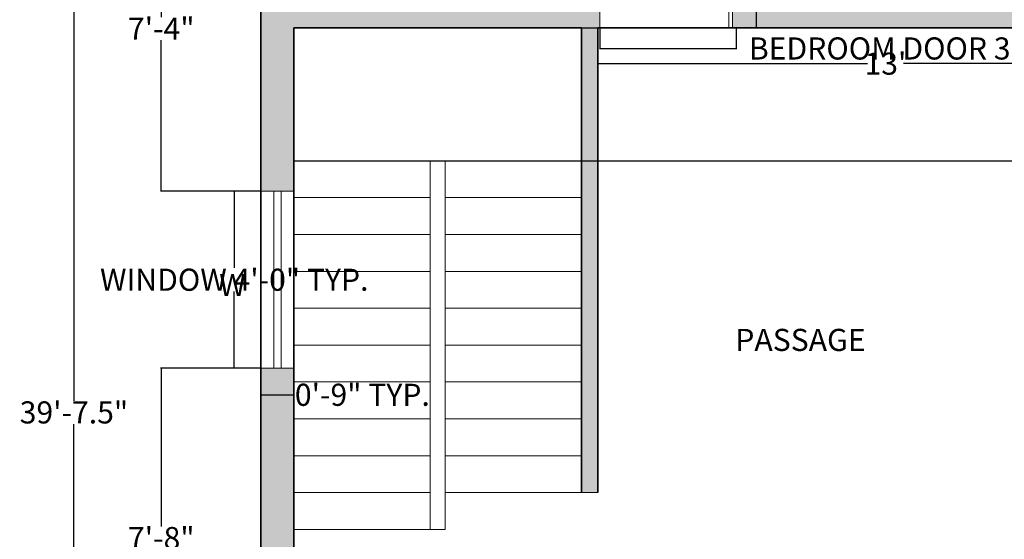
# Model space of a CAD drawing. Units: inches. Extents: x 302 to 1258, y 831 to 1373.
# Tile 2 of 13: x 302 to 569, y 1070 to 1211. Entities that reach past the tile are written whole.
import ezdxf

# ---------------------------------------------------------------- set-up
doc = ezdxf.new("R2010")
doc.units = ezdxf.units.IN
doc.header["$MEASUREMENT"] = 0
for name, color, linetype, lineweight in [('A-ANNO-DIMS', 2, 'Continuous', 18), ('A-ANNO-TEXT', 7, 'Continuous', 18), ('A-AREA-IDEN', 7, 'Continuous', 18), ('A-DOOR', 3, 'Continuous', 18), ('A-FLOR-STRS', 7, 'Continuous', 18), ('A-GLAZ', 4, 'Continuous', 18), ('A-WALL', 7, 'Continuous', 35), ('A-WALL-PATT', 251, 'Continuous', 13)]:
    doc.layers.add(name, color=color, linetype=linetype, lineweight=lineweight)
doc.styles.get("Standard").update_dxf_attribs({"font": 'arial.ttf'})
doc.dimstyles.get("Standard").update_dxf_attribs({"dimtxt": 6, "dimasz": 0.18, "dimexe": 0.18, "dimexo": 0.0625, "dimgap": 0.09, "dimtad": 0, "dimtih": 1, "dimtoh": 1, "dimdec": 1, "dimzin": 0, "dimdsep": 46, "dimlunit": 3, "dimtxsty": 'Standard', "dimcen": 0.09, "dimadec": 0, "dimazin": 0, "dimtfac": 1, "dimtdec": 1, "dimtofl": 0, "dimtmove": 0, "dimatfit": 3, "dimfxl": 1, "dimtolj": 1, "dimtzin": 0, "dimarcsym": 0})

# ---------------------------------------------------------------- blocks, each defined once
blk = doc.blocks.new('*D16')
at = {"layer": 'A-ANNO-DIMS', "color": 0, "lineweight": -2, "transparency": 16777216}
for p, q in [((459.17, 1208.76), (459.17, 1198.98)), ((615.17, 1208.76), (615.17, 1198.98)), ((459.35, 1199.16), (532.27, 1199.16)), ((614.99, 1199.16), (542.07, 1199.16))]:
    blk.add_line(p, q, dxfattribs=at)
at = {"layer": 'A-ANNO-DIMS', "color": 0, "transparency": 16777216}
for points in [[(459.35, 1199.19), (459.35, 1199.13), (459.17, 1199.16)], [(614.99, 1199.19), (614.99, 1199.13), (615.17, 1199.16)]]:
    blk.add_solid(points, dxfattribs=at)
at = {"layer": 'Defpoints', "color": 0, "transparency": 16777216}
for p in [(459.17, 1208.82), (615.17, 1208.82), (615.17, 1199.16)]:
    blk.add_point(p, dxfattribs=at)
at = {"layer": 'A-ANNO-DIMS', "color": 0, "transparency": 16777216, "insert": (537.17, 1199.16), "char_height": 6, "attachment_point": 5}
blk.add_mtext("\\A1;13'", dxfattribs=at)
blk = doc.blocks.new('*D32')
at = {"layer": 'A-ANNO-DIMS', "color": 0, "lineweight": -2, "transparency": 16777216}
for p, q in [((367.61, 1342.32), (316.79, 1342.32)), ((316.97, 1342.14), (316.97, 1107.72)), ((316.97, 867), (316.97, 1101.41)), ((367.61, 866.82), (316.79, 866.82))]:
    blk.add_line(p, q, dxfattribs=at)
at = {"layer": 'A-ANNO-DIMS', "color": 0, "transparency": 16777216}
for points in [[(316.94, 1342.14), (317, 1342.14), (316.97, 1342.32)], [(316.94, 867), (317, 867), (316.97, 866.82)]]:
    blk.add_solid(points, dxfattribs=at)
at = {"layer": 'Defpoints', "color": 0, "transparency": 16777216}
for p in [(367.67, 1342.32), (316.97, 866.82), (367.67, 866.82)]:
    blk.add_point(p, dxfattribs=at)
at = {"layer": 'A-ANNO-DIMS', "color": 0, "transparency": 16777216, "insert": (316.97, 1104.57), "char_height": 6, "attachment_point": 5}
blk.add_mtext('\\A1;39\'-7.5"', dxfattribs=at)
blk = doc.blocks.new('WINDOW-48IN')
for p, q in [((0, 0), (0, 9)), ((0, 9), (48, 9)), ((48, 9), (48, 0)), ((0, 5.5), (48, 5.5)), ((48, 3.5), (0, 3.5)), ((48, 0), (0, 0))]:
    blk.add_line(p, q)
blk = doc.blocks.new('DOOR-36IN-BEDROOM')
for p, q in [((35, 36), (35, 0)), ((36, 0), (36, 36)), ((36, 36), (36, 0)), ((0, 0), (0, 4.5)), ((36, 0), (0, 0)), ((37, 0), (36, 0))]:
    blk.add_line(p, q)
blk.add_arc((36, -0.32), 36.32, 90, 172.3719)
blk = doc.blocks.new('STAIR-RETURN-RUNS')
for p, q in [((0, 100), (78, 100)), ((37, 100), (37, 0)), ((41, 100), (41, 0)), ((0, 90), (37, 90)), ((41, 90), (78, 90)), ((0, 80), (37, 80)), ((41, 80), (78, 80)), ((0, 70), (37, 70)), ((41, 70), (78, 70)), ((0, 60), (37, 60)), ((41, 60), (78, 60)), ((0, 50), (37, 50)), ((41, 50), (78, 50)), ((0, 40), (37, 40)), ((41, 40), (78, 40)), ((0, 30), (37, 30)), ((41, 30), (78, 30)), ((0, 20), (37, 20)), ((41, 20), (78, 20)), ((0, 10), (37, 10)), ((41, 10), (82.5, 10)), ((0, 0), (41, 0))]:
    blk.add_line(p, q)
blk = doc.blocks.new('*D45')
at = {"layer": 'A-ANNO-DIMS', "color": 0, "lineweight": -2, "transparency": 16777216}
for p, q in [((367.61, 1164.55), (360.29, 1164.55)), ((360.47, 1164.37), (360.47, 1143.74)), ((360.47, 1116.73), (360.47, 1137.36)), ((367.61, 1116.55), (360.29, 1116.55))]:
    blk.add_line(p, q, dxfattribs=at)
at = {"layer": 'A-ANNO-DIMS', "color": 0, "transparency": 16777216}
for points in [[(360.44, 1164.37), (360.5, 1164.37), (360.47, 1164.55)], [(360.44, 1116.73), (360.5, 1116.73), (360.47, 1116.55)]]:
    blk.add_solid(points, dxfattribs=at)
at = {"layer": 'Defpoints', "color": 0, "transparency": 16777216}
for p in [(367.67, 1164.55), (360.47, 1116.55), (367.67, 1116.55)]:
    blk.add_point(p, dxfattribs=at)
at = {"layer": 'A-ANNO-DIMS', "color": 0, "transparency": 16777216, "insert": (360.47, 1140.55), "char_height": 6, "attachment_point": 5}
blk.add_mtext('\\A1;WINDOW 4\'-0" TYP.', dxfattribs=at)
blk = doc.blocks.new('*D46')
at = {"layer": 'A-ANNO-DIMS', "color": 0, "lineweight": -2, "transparency": 16777216}
for p, q in [((367.67, 1116.49), (367.67, 1109.17)), ((376.67, 1116.49), (376.67, 1109.17)), ((367.85, 1109.35), (376.49, 1109.35)), ((376.67, 1109.35), (376.85, 1109.35))]:
    blk.add_line(p, q, dxfattribs=at)
at = {"layer": 'A-ANNO-DIMS', "color": 0, "transparency": 16777216}
for points in [[(367.85, 1109.38), (367.85, 1109.32), (367.67, 1109.35)], [(376.49, 1109.38), (376.49, 1109.32), (376.67, 1109.35)]]:
    blk.add_solid(points, dxfattribs=at)
at = {"layer": 'Defpoints', "color": 0, "transparency": 16777216}
for p in [(367.67, 1116.55), (376.67, 1116.55), (376.67, 1109.35)]:
    blk.add_point(p, dxfattribs=at)
at = {"layer": 'A-ANNO-DIMS', "color": 0, "transparency": 16777216, "insert": (395.23, 1109.35), "char_height": 6, "attachment_point": 5}
blk.add_mtext('\\A1;0\'-9" TYP.', dxfattribs=at)
blk = doc.blocks.new('*D55')
at = {"layer": 'A-ANNO-DIMS', "color": 0, "lineweight": -2, "transparency": 16777216}
for p, q in [((459.67, 1208.76), (459.67, 1203.09)), ((496.67, 1208.76), (496.67, 1203.09)), ((459.85, 1203.27), (496.49, 1203.27)), ((496.67, 1203.27), (496.85, 1203.27))]:
    blk.add_line(p, q, dxfattribs=at)
at = {"layer": 'A-ANNO-DIMS', "color": 0, "transparency": 16777216}
for points in [[(459.85, 1203.3), (459.85, 1203.24), (459.67, 1203.27)], [(496.49, 1203.3), (496.49, 1203.24), (496.67, 1203.27)]]:
    blk.add_solid(points, dxfattribs=at)
at = {"layer": 'Defpoints', "color": 0, "transparency": 16777216}
for p in [(459.67, 1208.82), (496.67, 1208.82), (496.67, 1203.27)]:
    blk.add_point(p, dxfattribs=at)
at = {"layer": 'A-ANNO-DIMS', "color": 0, "transparency": 16777216, "insert": (551.65, 1203.27), "char_height": 6, "attachment_point": 5}
blk.add_mtext('\\A1;BEDROOM DOOR 3\'-1" TYP.', dxfattribs=at)
blk = doc.blocks.new('*D56')
at = {"layer": 'A-ANNO-DIMS', "color": 0, "lineweight": -2, "transparency": 16777216}
for p, q in [((496.73, 1244.82), (502.4, 1244.82)), ((502.22, 1244.64), (502.22, 1229.97)), ((502.22, 1209), (502.22, 1223.66)), ((496.73, 1208.82), (502.4, 1208.82))]:
    blk.add_line(p, q, dxfattribs=at)
at = {"layer": 'A-ANNO-DIMS', "color": 0, "transparency": 16777216}
for points in [[(502.19, 1244.64), (502.25, 1244.64), (502.22, 1244.82)], [(502.19, 1209), (502.25, 1209), (502.22, 1208.82)]]:
    blk.add_solid(points, dxfattribs=at)
at = {"layer": 'Defpoints', "color": 0, "transparency": 16777216}
for p in [(496.67, 1244.82), (502.22, 1244.82), (496.67, 1208.82)]:
    blk.add_point(p, dxfattribs=at)
at = {"layer": 'A-ANNO-DIMS', "color": 0, "transparency": 16777216, "insert": (502.22, 1226.82), "char_height": 6, "attachment_point": 5}
blk.add_mtext('\\A1;3\'-0" TYP.', dxfattribs=at)
blk = doc.blocks.new('*D72')
at = {"layer": 'A-ANNO-DIMS', "color": 0, "lineweight": -2, "transparency": 16777216}
for p, q in [((367.60766, 1252.758966), (340.49016, 1252.758966)), ((340.67016, 1252.578966), (340.67016, 1211.744211)), ((340.67016, 1164.729456), (340.67016, 1205.564211)), ((367.60766, 1164.549456), (340.49016, 1164.549456))]:
    blk.add_line(p, q, dxfattribs=at)
at = {"layer": 'A-ANNO-DIMS', "color": 0, "transparency": 16777216}
for points in [[(340.64016, 1252.578966), (340.70016, 1252.578966), (340.67016, 1252.758966)], [(340.64016, 1164.729456), (340.70016, 1164.729456), (340.67016, 1164.549456)]]:
    blk.add_solid(points, dxfattribs=at)
at = {"layer": 'Defpoints', "color": 0, "transparency": 16777216}
for p in [(367.67016, 1252.758966), (340.67016, 1164.549456), (367.67016, 1164.549456)]:
    blk.add_point(p, dxfattribs=at)
at = {"layer": 'A-ANNO-DIMS', "color": 0, "transparency": 16777216, "insert": (340.67016, 1208.654211), "char_height": 6, "attachment_point": 5}
blk.add_mtext('\\A1;7\'-4"', dxfattribs=at)
blk = doc.blocks.new('*D73')
at = {"layer": 'A-ANNO-DIMS', "color": 0, "lineweight": -2, "transparency": 16777216}
for p, q in [((367.61, 1116.55), (340.49, 1116.55)), ((340.67, 1116.37), (340.67, 1073.65)), ((340.67, 1024.62), (340.67, 1067.34)), ((367.61, 1024.44), (340.49, 1024.44))]:
    blk.add_line(p, q, dxfattribs=at)
at = {"layer": 'A-ANNO-DIMS', "color": 0, "transparency": 16777216}
for points in [[(340.64, 1116.37), (340.7, 1116.37), (340.67, 1116.55)], [(340.64, 1024.62), (340.7, 1024.62), (340.67, 1024.44)]]:
    blk.add_solid(points, dxfattribs=at)
at = {"layer": 'Defpoints', "color": 0, "transparency": 16777216}
for p in [(367.67, 1116.55), (340.67, 1024.44), (367.67, 1024.44)]:
    blk.add_point(p, dxfattribs=at)
at = {"layer": 'A-ANNO-DIMS', "color": 0, "transparency": 16777216, "insert": (340.67, 1070.49), "char_height": 6, "attachment_point": 5}
blk.add_mtext('\\A1;7\'-8"', dxfattribs=at)
blk = doc.blocks.new('*D83')
at = {"layer": 'A-ANNO-DIMS', "color": 0, "lineweight": -2, "transparency": 16777216}
for p, q in [((376.73, 1208.82), (751.85, 1208.82)), ((751.67, 1208.64), (751.67, 1193.97)), ((751.67, 1173), (751.67, 1187.66)), ((376.73, 1172.82), (751.85, 1172.82))]:
    blk.add_line(p, q, dxfattribs=at)
at = {"layer": 'A-ANNO-DIMS', "color": 0, "transparency": 16777216}
for points in [[(751.64, 1208.64), (751.7, 1208.64), (751.67, 1208.82)], [(751.64, 1173), (751.7, 1173), (751.67, 1172.82)]]:
    blk.add_solid(points, dxfattribs=at)
at = {"layer": 'Defpoints', "color": 0, "transparency": 16777216}
for p in [(376.67, 1208.82), (751.67, 1208.82), (376.67, 1172.82)]:
    blk.add_point(p, dxfattribs=at)
at = {"layer": 'A-ANNO-DIMS', "color": 0, "transparency": 16777216, "insert": (751.67, 1190.82), "char_height": 6, "attachment_point": 5}
blk.add_mtext('\\A1;3\'-0"', dxfattribs=at)

msp = doc.modelspace()

# ---------------------------------------------------------------- hatches: boundary and pattern name
at = {"layer": 'A-WALL-PATT'}
h = msp.add_hatch(color=256, dxfattribs=at)
h.dxf.hatch_style = 1
h.paths.add_polyline_path([(524.78, 1342.32), (455.57, 1342.32), (455.57, 1333.32), (496.67, 1333.32), (496.67, 1330.32), (501.17, 1330.32), (501.17, 1333.32), (524.78, 1333.32)])
h.paths.add_polyline_path([(724.67, 1342.32), (548.78, 1342.32), (548.78, 1333.32), (567.17, 1333.32), (567.17, 1213.32), (501.17, 1213.32), (501.17, 1306.32), (496.67, 1306.32), (496.67, 1213.32), (495.67, 1213.32), (495.67, 1208.82), (496.67, 1208.82), (572.67, 1208.82), (572.67, 1213.32), (571.67, 1213.32), (571.67, 1333.32), (715.67, 1333.32), (715.67, 1302.71), (724.67, 1302.71)])
h.paths.add_polyline_path([(376.67, 1333.32), (407.57, 1333.32), (407.57, 1342.32), (367.67, 1342.32), (367.67, 1300.76), (376.67, 1300.76)])
h.paths.add_polyline_path([(459.67, 1213.32), (376.67, 1213.32), (376.67, 1252.76), (367.67, 1252.76), (367.67, 1164.55), (376.67, 1164.55), (376.67, 1208.82), (454.67, 1208.82), (454.67, 1082.82), (459.17, 1082.82), (459.17, 1208.82), (459.67, 1208.82)])
h.paths.add_polyline_path([(376.67, 1116.55), (367.67, 1116.55), (367.67, 1024.44), (376.67, 1024.44)])
h.paths.add_polyline_path([(724.67, 1254.71), (715.67, 1254.71), (715.67, 1213.32), (608.67, 1213.32), (608.67, 1208.82), (615.17, 1208.82), (615.17, 1205.82), (619.67, 1205.82), (619.67, 1208.82), (715.67, 1208.82), (715.67, 1191.3), (724.67, 1191.3)])
h.paths.add_polyline_path([(724.67, 1167.3), (715.67, 1167.3), (715.67, 1136.82), (619.67, 1136.82), (619.67, 1181.82), (615.17, 1181.82), (615.17, 1136.82), (591.17, 1136.82), (591.17, 1129.32), (595.67, 1129.32), (595.67, 1132.32), (715.67, 1132.32), (715.67, 1097.42), (724.67, 1097.42)])
h.paths.add_polyline_path([(724.67, 1049.42), (715.67, 1049.42), (715.67, 1012.32), (595.67, 1012.32), (595.67, 1093.32), (591.17, 1093.32), (591.17, 1007.82), (715.67, 1007.82), (715.67, 875.82), (709.67, 875.82), (709.67, 866.82), (715.67, 866.82), (724.67, 866.82)])
h.paths.add_polyline_path([(673.67, 875.82), (623.88, 875.82), (623.88, 866.82), (673.67, 866.82)], flags=17)
h.paths.add_polyline_path([(575.88, 875.82), (477.17, 875.82), (477.17, 971.82), (472.67, 971.82), (472.67, 875.82), (376.67, 875.82), (376.67, 896.2), (367.67, 896.2), (367.67, 866.82), (575.88, 866.82)])
h.paths.add_polyline_path([(376.67, 976.44), (367.67, 976.44), (367.67, 944.2), (376.67, 944.2)])

# ---------------------------------------------------------------- linework, layer by layer
at = {"layer": 'A-WALL'}
for p, q in [((367.67, 1342.32), (367.67, 866.82)), ((376.67, 1208.82), (454.67, 1208.82)), ((376.67, 1208.82), (376.67, 875.82)), ((454.67, 1208.82), (454.67, 1082.82)), ((459.17, 1208.82), (459.17, 1082.82)), ((459.17, 1208.82), (615.17, 1208.82))]:
    msp.add_line(p, q, dxfattribs=at)

# ---------------------------------------------------------------- block references
at = {"layer": 'A-DOOR'}
msp.add_blockref('DOOR-36IN-BEDROOM', (459.67, 1208.82), dxfattribs=at)
at = {"layer": 'A-FLOR-STRS'}
msp.add_blockref('STAIR-RETURN-RUNS', (376.67, 1072.82), dxfattribs=at)
at = {"layer": 'A-GLAZ', "rotation": 269.9999999999994}
msp.add_blockref('WINDOW-48IN', (367.67, 1164.55), dxfattribs=at)

# ---------------------------------------------------------------- texts
at = {"layer": 'A-ANNO-TEXT', "insert": (356.39, 1142.12), "char_height": 6, "attachment_point": 1}
msp.add_mtext_dynamic_manual_height_columns('W', width=16.4894, gutter_width=30, heights=[0], dxfattribs=at)
at = {"layer": 'A-AREA-IDEN', "insert": (496.43, 1127.23), "char_height": 6, "attachment_point": 1}
msp.add_mtext_dynamic_manual_height_columns('PASSAGE', width=60.5592, gutter_width=30, heights=[0], dxfattribs=at)

# ---------------------------------------------------------------- dimensions: what is measured, and where the dimension line sits
at = {"layer": 'A-ANNO-DIMS'}
for base, p1, p2, override, picture, middle in [((316.97, 866.82), (367.67, 1342.32), (367.67, 866.82), {"dimclrd": 0, "dimclre": 0, "dimclrt": 0}, '*D32', (316.97, 1104.57)), ((340.67, 1164.55), (367.67, 1252.76), (367.67, 1164.55), {"dimdec": 1, "dimlfac": 1, "dimrnd": 0, "dimzin": 1, "dimdsep": 46, "dimlunit": 4, "dimfrac": 2}, '*D72', (340.67, 1208.65)), ((751.67, 1208.82), (376.67, 1172.82), (376.67, 1208.82), {"dimdec": 1, "dimlfac": 1, "dimrnd": 0, "dimzin": 1, "dimdsep": 46, "dimlunit": 4, "dimfrac": 2}, '*D83', (751.67, 1190.82)), ((340.67, 1024.44), (367.67, 1116.55), (367.67, 1024.44), {"dimdec": 1, "dimlfac": 1, "dimrnd": 0, "dimzin": 1, "dimdsep": 46, "dimlunit": 4, "dimfrac": 2}, '*D73', (340.67, 1070.49))]:
    dim = msp.add_linear_dim(base=base, p1=p1, p2=p2, angle=90, dimstyle='Standard', override=override, dxfattribs=at)
    dim.commit()
    dim.dimension.update_dxf_attribs({"geometry": picture, "text_midpoint": middle})
for base, p1, p2, angle, text, picture, middle in [((502.22, 1244.82), (496.67, 1208.82), (496.67, 1244.82), 90, '<> TYP.', '*D56', (502.22, 1226.82)), ((360.47, 1116.55), (367.67, 1164.55), (367.67, 1116.55), 270, 'WINDOW <> TYP.', '*D45', (360.47, 1140.55))]:
    dim = msp.add_linear_dim(base=base, p1=p1, p2=p2, angle=angle, text=text, dimstyle='Standard', override={"dimdec": 1, "dimlfac": 1, "dimrnd": 0, "dimzin": 1, "dimdsep": 46, "dimlunit": 4, "dimfrac": 2}, dxfattribs=at)
    dim.commit()
    dim.dimension.update_dxf_attribs({"geometry": picture, "text_midpoint": middle})
for base, p1, p2, text, picture, middle in [((496.67, 1203.27), (459.67, 1208.82), (496.67, 1208.82), 'BEDROOM DOOR <> TYP.', '*D55', (551.65, 1203.27)), ((376.67, 1109.35), (367.67, 1116.55), (376.67, 1116.55), '<> TYP.', '*D46', (395.23, 1109.35))]:
    dim = msp.add_linear_dim(base=base, p1=p1, p2=p2, text=text, dimstyle='Standard', override={"dimdec": 1, "dimlfac": 1, "dimrnd": 0, "dimzin": 1, "dimdsep": 46, "dimlunit": 4, "dimfrac": 2}, dxfattribs=at)
    dim.commit()
    dim.dimension.update_dxf_attribs({"geometry": picture, "text_midpoint": middle})
dim = msp.add_linear_dim(base=(615.17, 1199.16), p1=(459.17, 1208.82), p2=(615.17, 1208.82), dimstyle='Standard', override={"dimclrd": 0, "dimclre": 0, "dimclrt": 0}, dxfattribs=at)
dim.commit()
dim.dimension.update_dxf_attribs({"geometry": '*D16', "text_midpoint": (537.17, 1199.16)})

doc.saveas('drawing.dxf')
